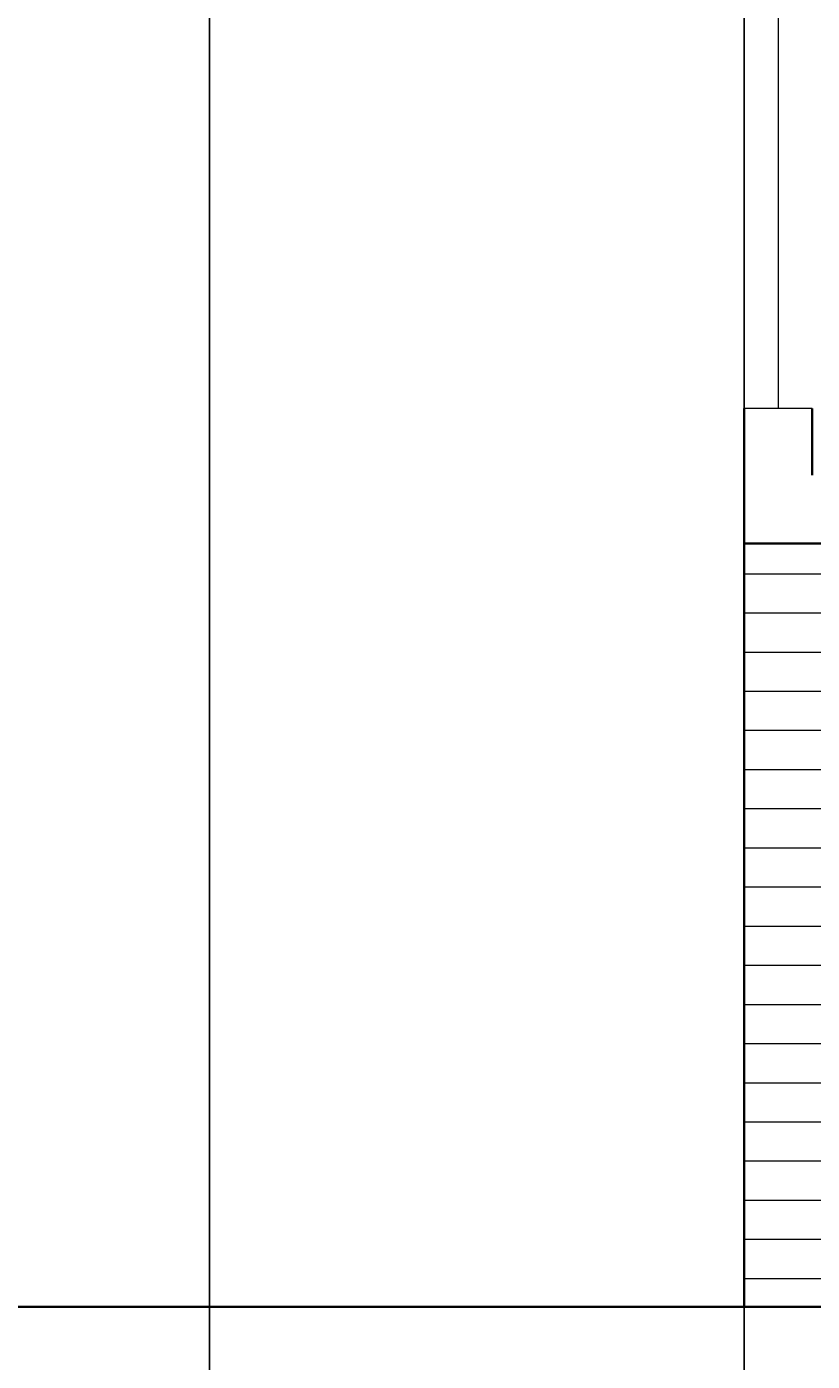
# Model space of a CAD drawing. Units: inches. Extents: x 1088 to 1703, y 668 to 1875.
# Tile 26 of 45: x 1539 to 1590, y 1416 to 1504. Entities that reach past the tile are written whole.
import ezdxf

# ---------------------------------------------------------------- set-up
doc = ezdxf.new("R2010")
doc.units = ezdxf.units.IN
for name, color, linetype, lineweight in [('A-ANNO-DIMS', 2, 'Continuous', 18), ('A-DOOR', 4, 'Continuous', 18), ('A-FLOR-PATT', 252, 'Continuous', 13), ('A-WALL', 7, 'Continuous', 35)]:
    doc.layers.add(name, color=color, linetype=linetype, lineweight=lineweight)
doc.styles.get("Standard").update_dxf_attribs({"font": 'arial.ttf'})
doc.dimstyles.get("Standard").update_dxf_attribs({"dimtxt": 0.18, "dimasz": 0.18, "dimexe": 0.18, "dimexo": 0.0625, "dimgap": 0.09, "dimtad": 0, "dimtih": 1, "dimtoh": 1, "dimdec": 4, "dimzin": 0, "dimdsep": 46, "dimtxsty": 'Standard', "dimcen": 0.09, "dimadec": 0, "dimazin": 0, "dimtfac": 1, "dimtdec": 4, "dimtofl": 0, "dimtmove": 0, "dimatfit": 3, "dimfxl": 1, "dimtolj": 1, "dimtzin": 0, "dimarcsym": 0})

# ---------------------------------------------------------------- blocks, each defined once
blk = doc.blocks.new('*D32')
at = {"layer": 'A-ANNO-DIMS', "color": 0, "lineweight": -2, "transparency": 16777216}
for p, q in [((1550.595, 1373.121), (1550.595, 1857.788)), ((1550.775, 1857.608), (1567.825, 1857.608)), ((1585.665, 1857.608), (1568.614, 1857.608)), ((1585.845, 1360.983), (1585.845, 1857.788))]:
    blk.add_line(p, q, dxfattribs=at)
at = {"layer": 'A-ANNO-DIMS', "color": 0, "transparency": 16777216}
for points in [[(1550.775, 1857.638), (1550.775, 1857.578), (1550.595, 1857.608)], [(1585.665, 1857.638), (1585.665, 1857.578), (1585.845, 1857.608)]]:
    blk.add_solid(points, dxfattribs=at)
at = {"layer": 'Defpoints', "color": 0, "transparency": 16777216}
for p in [(1585.845, 1857.608), (1550.595, 1373.058), (1585.845, 1360.921)]:
    blk.add_point(p, dxfattribs=at)
at = {"layer": 'A-ANNO-DIMS', "color": 0, "transparency": 16777216, "insert": (1568.22, 1857.608), "char_height": 0.18, "attachment_point": 5}
blk.add_mtext('\\A1;35.25', dxfattribs=at)

msp = doc.modelspace()

# ---------------------------------------------------------------- hatches: boundary and pattern name
at = {"layer": 'A-FLOR-PATT'}
h = msp.add_hatch(dxfattribs=at)
h.set_pattern_fill('ANSI31', color=256, scale=0.812516, angle=-45, style=0)
h.paths.add_polyline_path([(1585.845, 1419.558), (1615.845, 1419.558), (1615.845, 1469.863), (1585.845, 1469.863)])

# ---------------------------------------------------------------- linework, layer by layer
at = {"layer": 'A-DOOR'}
for p, q in [((1588.095, 1539.558), (1588.095, 1478.749)), ((1590.345, 1478.749), (1585.845, 1478.749))]:
    msp.add_line(p, q, dxfattribs=at)
at = {"layer": 'A-WALL'}
for p, q in [((1585.845, 1478.749), (1585.845, 1419.558)), ((1590.345, 1478.749), (1590.345, 1474.363)), ((1585.845, 1474.363), (1585.845, 1469.863)), ((1615.845, 1469.863), (1585.845, 1469.863)), ((1585.845, 1419.558), (1440.345, 1419.558)), ((1485.345, 1419.558), (1585.845, 1419.558)), ((1615.845, 1419.558), (1585.845, 1419.558))]:
    msp.add_line(p, q, dxfattribs=at)

# ---------------------------------------------------------------- dimensions: what is measured, and where the dimension line sits
at = {"layer": 'A-ANNO-DIMS'}
dim = msp.add_linear_dim(base=(1585.845, 1857.608), p1=(1550.595, 1373.058), p2=(1585.845, 1360.921), dimstyle='Standard', override={"dimdec": 2, "dimlfac": 1, "dimrnd": 0, "dimzin": 0, "dimdsep": 46, "dimlunit": 2}, dxfattribs=at)
dim.commit()
dim.dimension.update_dxf_attribs({"geometry": '*D32', "text_midpoint": (1568.22, 1857.608)})

doc.saveas('drawing.dxf')
